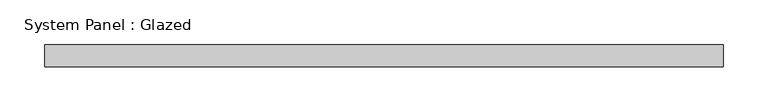
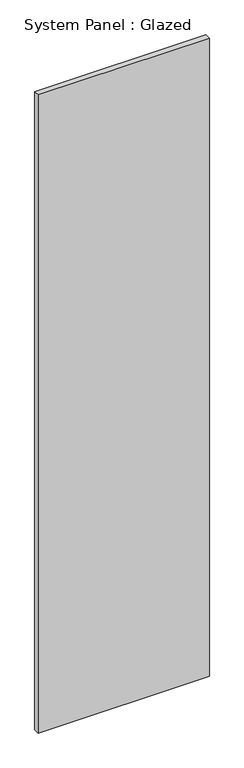
"""IFC4 building model written with IfcOpenShell, lengths in millimetres: plate geometry, System Panel : Glazed."""

from ifc_helpers import new_model, si_unit, origin, origin_with_axes, place, context, project, spatial, polyline, outline, extrude, source, transform, mapped, element, save


def system_panel_glazed_bd0dc997(model_context):
    return source(origin(), model_context, "Body", "SweptSolid", [
        extrude(outline(polyline([(381.0, 24.5), (-381.0, 24.5), (-381.0, 49.5), (381.0, 49.5), (381.0, 24.5)])), origin_with_axes(), (0.0, 0.0, 1.0), 3000.0),
    ])


if __name__ == "__main__":
    model = new_model("IFC4")
    model_context = context("Model", 3, world=origin())
    ifc_project = project(units=[si_unit("LENGTHUNIT", "METRE", prefix="MILLI")], contexts=[model_context])
    site = spatial("IfcSite", under=ifc_project)
    building = spatial("IfcBuilding", under=site)
    placement = place(None, origin())
    system_panel_glazed_shape = system_panel_glazed_bd0dc997(model_context)
    element("IfcPlate", 1, ObjectType="System Panel : Glazed", at=placement, inside=building, context=model_context, shape_type="MappedRepresentation", body=[
        mapped(system_panel_glazed_shape, transform((0.0, 0.0, 0.0), x_axis=(1.0, 0.0, 0.0), y_axis=(0.0, 1.0, 0.0), z_axis=(0.0, 0.0, 1.0))),
    ])
    save(model, "model.ifc")

# Revit data of these elements
# Type "System Panel : Glazed"
#   Keynote = "H11"
#   Construction Type Id = "GSP4R"
#   Analytic Construction = "1/8 in Pilkington single glazing"
#   Visual Light Transmittance = 0.9
#   Solar Heat Gain Coefficient = 0.86
#   Heat Transfer Coefficient (U) = 6.7069 W/(m²·K)
#   Define Thermal Properties by = 1
# Element 1 (IfcPlate, "System Panel : Glazed")
#   Materials on its faces: "Glass"
# Materials
#   "Glass": class "Glass", colour RGB 0 128 192, transparency 0.9, Description = "Soda Lime Glass", Cost = 0
